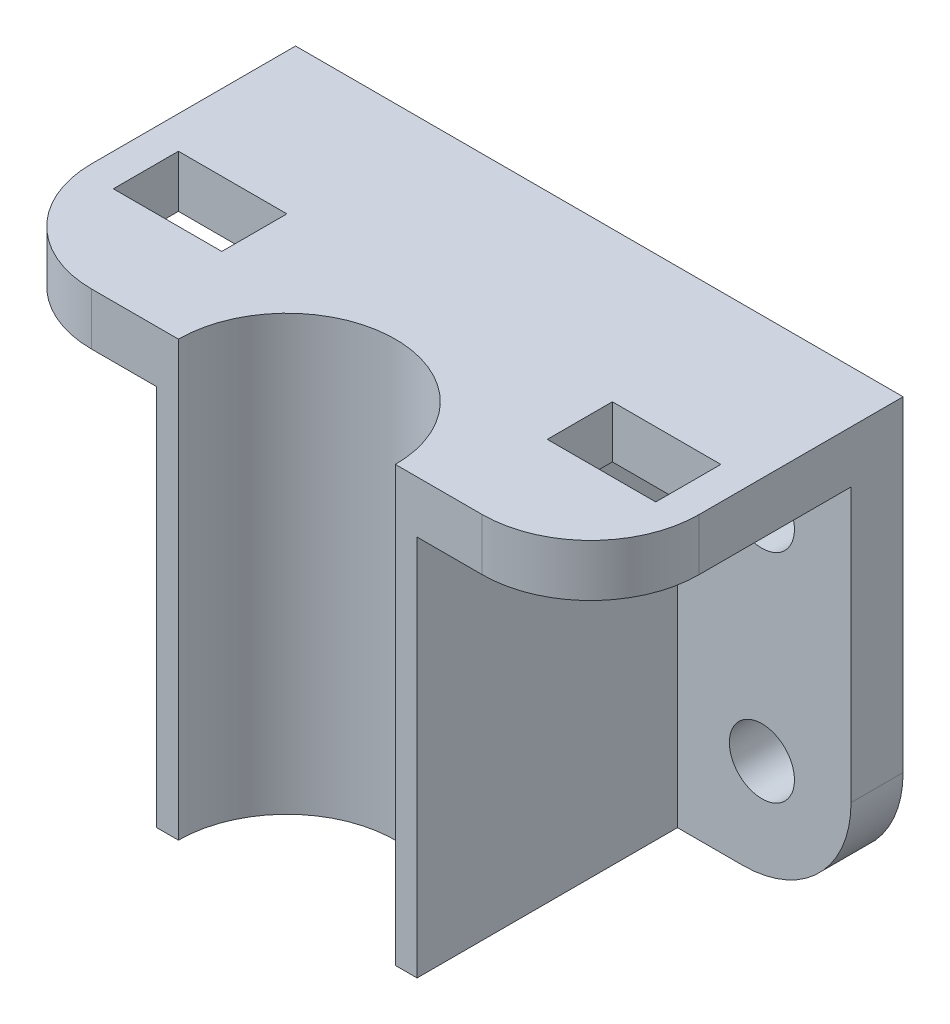
ISO-10303-21;
HEADER;
FILE_DESCRIPTION(('STEP AP214'),'2;1');
FILE_NAME('part.step','',(''),(''),'','','');
FILE_SCHEMA(('AUTOMOTIVE_DESIGN { 1 0 10303 214 1 1 1 1 }'));
ENDSEC;
DATA;
#1=APPLICATION_CONTEXT('core data for automotive mechanical design processes');
#2=APPLICATION_PROTOCOL_DEFINITION('international standard','automotive_design',2000,#1);
#3=PRODUCT_CONTEXT('',#1,'mechanical');
#4=PRODUCT('Part','Part','',(#3));
#5=PRODUCT_RELATED_PRODUCT_CATEGORY('part','',(#4));
#6=PRODUCT_DEFINITION_FORMATION('','',#4);
#7=PRODUCT_DEFINITION_CONTEXT('part definition',#1,'design');
#8=PRODUCT_DEFINITION('design','',#6,#7);
#9=PRODUCT_DEFINITION_SHAPE('','',#8);
#10=(LENGTH_UNIT() NAMED_UNIT(*) SI_UNIT(.MILLI.,.METRE.));
#11=(NAMED_UNIT(*) PLANE_ANGLE_UNIT() SI_UNIT($,.RADIAN.));
#12=(NAMED_UNIT(*) SI_UNIT($,.STERADIAN.) SOLID_ANGLE_UNIT());
#13=UNCERTAINTY_MEASURE_WITH_UNIT(LENGTH_MEASURE(1.E-05),#10,'distance_accuracy_value','');
#14=(GEOMETRIC_REPRESENTATION_CONTEXT(3) GLOBAL_UNCERTAINTY_ASSIGNED_CONTEXT((#13)) GLOBAL_UNIT_ASSIGNED_CONTEXT((#10,
#11,#12)) REPRESENTATION_CONTEXT('',''));
#15=CARTESIAN_POINT('',(0.,0.,0.));
#16=DIRECTION('',(0.,0.,1.));
#17=DIRECTION('',(1.,0.,0.));
#18=AXIS2_PLACEMENT_3D('',#15,#16,#17);
#19=CARTESIAN_POINT('',(115.,-12.,72.));
#20=DIRECTION('',(0.,0.,1.));
#21=DIRECTION('',(1.,0.,0.));
#22=AXIS2_PLACEMENT_3D('',#19,#20,#21);
#23=PLANE('',#22);
#24=DIRECTION('',(0.,1.,0.));
#25=VECTOR('',#24,1.);
#26=CARTESIAN_POINT('',(45.0000000000001,-100.,72.));
#27=LINE('',#26,#25);
#28=CARTESIAN_POINT('',(45.0000000000001,-100.,72.));
#29=VERTEX_POINT('',#28);
#30=CARTESIAN_POINT('',(45.0000000000001,0.,72.));
#31=VERTEX_POINT('',#30);
#32=EDGE_CURVE('E303',#29,#31,#27,.T.);
#33=ORIENTED_EDGE('',*,*,#32,.T.);
#34=DIRECTION('',(1.,0.,0.));
#35=VECTOR('',#34,1.);
#36=CARTESIAN_POINT('',(115.,0.,72.));
#37=LINE('',#36,#35);
#38=CARTESIAN_POINT('',(25.,0.,72.));
#39=VERTEX_POINT('',#38);
#40=EDGE_CURVE('E336',#39,#31,#37,.T.);
#41=ORIENTED_EDGE('',*,*,#40,.F.);
#42=DIRECTION('',(0.,1.,0.));
#43=VECTOR('',#42,1.);
#44=CARTESIAN_POINT('',(25.,-12.,72.));
#45=LINE('',#44,#43);
#46=CARTESIAN_POINT('',(25.,-12.,72.));
#47=VERTEX_POINT('',#46);
#48=EDGE_CURVE('E351',#47,#39,#45,.T.);
#49=ORIENTED_EDGE('',*,*,#48,.F.);
#50=DIRECTION('',(1.,0.,0.));
#51=VECTOR('',#50,1.);
#52=CARTESIAN_POINT('',(115.,-12.,72.));
#53=LINE('',#52,#51);
#54=CARTESIAN_POINT('',(40.0000000000001,-12.,72.));
#55=VERTEX_POINT('',#54);
#56=EDGE_CURVE('E323',#47,#55,#53,.T.);
#57=ORIENTED_EDGE('',*,*,#56,.T.);
#58=DIRECTION('',(0.,1.,0.));
#59=VECTOR('',#58,1.);
#60=CARTESIAN_POINT('',(40.0000000000001,-100.,72.));
#61=LINE('',#60,#59);
#62=CARTESIAN_POINT('',(40.0000000000001,-100.,72.));
#63=VERTEX_POINT('',#62);
#64=EDGE_CURVE('E297',#63,#55,#61,.T.);
#65=ORIENTED_EDGE('',*,*,#64,.F.);
#66=DIRECTION('',(-1.,0.,0.));
#67=VECTOR('',#66,1.);
#68=CARTESIAN_POINT('',(45.0000000000001,-100.,72.));
#69=LINE('',#68,#67);
#70=EDGE_CURVE('E289',#29,#63,#69,.T.);
#71=ORIENTED_EDGE('',*,*,#70,.F.);
#72=EDGE_LOOP('',(#33,#41,#49,#57,#65,#71));
#73=FACE_BOUND('',#72,.T.);
#74=ADVANCED_FACE('F44',(#73),#23,.T.);
#75=CARTESIAN_POINT('',(115.,-75.,12.));
#76=DIRECTION('',(0.,0.,1.));
#77=DIRECTION('',(1.,0.,0.));
#78=AXIS2_PLACEMENT_3D('',#75,#76,#77);
#79=PLANE('',#78);
#80=CARTESIAN_POINT('',(119.4631545479,-27.,12.));
#81=DIRECTION('',(0.,0.,1.));
#82=DIRECTION('',(1.,0.,0.));
#83=AXIS2_PLACEMENT_3D('',#80,#81,#82);
#84=CIRCLE('',#83,7.49999999999998);
#85=CARTESIAN_POINT('',(126.9631545479,-27.,12.));
#86=VERTEX_POINT('',#85);
#87=EDGE_CURVE('E567',#86,#86,#84,.T.);
#88=ORIENTED_EDGE('',*,*,#87,.F.);
#89=EDGE_LOOP('',(#88));
#90=FACE_BOUND('',#89,.T.);
#91=CARTESIAN_POINT('',(119.4631545479,-77.,12.));
#92=DIRECTION('',(0.,0.,1.));
#93=DIRECTION('',(1.,0.,0.));
#94=AXIS2_PLACEMENT_3D('',#91,#92,#93);
#95=CIRCLE('',#94,7.50000000000001);
#96=CARTESIAN_POINT('',(126.9631545479,-77.,12.));
#97=VERTEX_POINT('',#96);
#98=EDGE_CURVE('E230',#97,#97,#95,.T.);
#99=ORIENTED_EDGE('',*,*,#98,.F.);
#100=EDGE_LOOP('',(#99));
#101=FACE_BOUND('',#100,.T.);
#102=DIRECTION('',(-1.,0.,0.));
#103=VECTOR('',#102,1.);
#104=CARTESIAN_POINT('',(140.,-12.,12.));
#105=LINE('',#104,#103);
#106=CARTESIAN_POINT('',(140.,-12.,12.));
#107=VERTEX_POINT('',#106);
#108=CARTESIAN_POINT('',(100.,-12.,12.));
#109=VERTEX_POINT('',#108);
#110=EDGE_CURVE('E313',#107,#109,#105,.T.);
#111=ORIENTED_EDGE('',*,*,#110,.T.);
#112=DIRECTION('',(0.,1.,0.));
#113=VECTOR('',#112,1.);
#114=CARTESIAN_POINT('',(100.,-100.,12.));
#115=LINE('',#114,#113);
#116=CARTESIAN_POINT('',(100.,-100.,12.));
#117=VERTEX_POINT('',#116);
#118=EDGE_CURVE('E309',#117,#109,#115,.T.);
#119=ORIENTED_EDGE('',*,*,#118,.F.);
#120=DIRECTION('',(1.,0.,0.));
#121=VECTOR('',#120,1.);
#122=CARTESIAN_POINT('',(25.,-100.,12.));
#123=LINE('',#122,#121);
#124=CARTESIAN_POINT('',(115.,-100.,12.));
#125=VERTEX_POINT('',#124);
#126=EDGE_CURVE('E359',#117,#125,#123,.T.);
#127=ORIENTED_EDGE('',*,*,#126,.T.);
#128=CARTESIAN_POINT('',(115.,-75.,12.));
#129=DIRECTION('',(0.,0.,1.));
#130=DIRECTION('',(1.,0.,0.));
#131=AXIS2_PLACEMENT_3D('',#128,#129,#130);
#132=CIRCLE('',#131,25.);
#133=CARTESIAN_POINT('',(140.,-75.,12.));
#134=VERTEX_POINT('',#133);
#135=EDGE_CURVE('E361',#125,#134,#132,.T.);
#136=ORIENTED_EDGE('',*,*,#135,.T.);
#137=DIRECTION('',(0.,1.,0.));
#138=VECTOR('',#137,1.);
#139=CARTESIAN_POINT('',(140.,0.,12.));
#140=LINE('',#139,#138);
#141=EDGE_CURVE('E362',#134,#107,#140,.T.);
#142=ORIENTED_EDGE('',*,*,#141,.T.);
#143=EDGE_LOOP('',(#111,#119,#127,#136,#142));
#144=FACE_BOUND('',#143,.T.);
#145=ADVANCED_FACE('F416',(#90,#101,#144),#79,.T.);
#146=CARTESIAN_POINT('',(19.128084721305,-27.,12.));
#147=DIRECTION('',(0.,0.,1.));
#148=DIRECTION('',(1.,0.,0.));
#149=AXIS2_PLACEMENT_3D('',#146,#147,#148);
#150=CIRCLE('',#149,7.5);
#151=CARTESIAN_POINT('',(26.628084721305,-27.,12.));
#152=VERTEX_POINT('',#151);
#153=EDGE_CURVE('E558',#152,#152,#150,.T.);
#154=ORIENTED_EDGE('',*,*,#153,.F.);
#155=EDGE_LOOP('',(#154));
#156=FACE_BOUND('',#155,.T.);
#157=CARTESIAN_POINT('',(19.128084721305,-77.,12.));
#158=DIRECTION('',(0.,0.,1.));
#159=DIRECTION('',(1.,0.,0.));
#160=AXIS2_PLACEMENT_3D('',#157,#158,#159);
#161=CIRCLE('',#160,7.5);
#162=CARTESIAN_POINT('',(26.628084721305,-77.,12.));
#163=VERTEX_POINT('',#162);
#164=EDGE_CURVE('E565',#163,#163,#161,.T.);
#165=ORIENTED_EDGE('',*,*,#164,.F.);
#166=EDGE_LOOP('',(#165));
#167=FACE_BOUND('',#166,.T.);
#168=CARTESIAN_POINT('',(25.,-100.,12.));
#169=VERTEX_POINT('',#168);
#170=CARTESIAN_POINT('',(40.0000000000001,-100.,12.));
#171=VERTEX_POINT('',#170);
#172=EDGE_CURVE('E363',#169,#171,#123,.T.);
#173=ORIENTED_EDGE('',*,*,#172,.T.);
#174=DIRECTION('',(0.,1.,0.));
#175=VECTOR('',#174,1.);
#176=CARTESIAN_POINT('',(40.0000000000001,-100.,12.));
#177=LINE('',#176,#175);
#178=CARTESIAN_POINT('',(40.0000000000001,-12.,12.));
#179=VERTEX_POINT('',#178);
#180=EDGE_CURVE('E291',#171,#179,#177,.T.);
#181=ORIENTED_EDGE('',*,*,#180,.T.);
#182=CARTESIAN_POINT('',(0.,-12.,12.));
#183=VERTEX_POINT('',#182);
#184=EDGE_CURVE('E319',#179,#183,#105,.T.);
#185=ORIENTED_EDGE('',*,*,#184,.T.);
#186=DIRECTION('',(0.,-1.,0.));
#187=VECTOR('',#186,1.);
#188=CARTESIAN_POINT('',(0.,0.,12.));
#189=LINE('',#188,#187);
#190=CARTESIAN_POINT('',(0.,-75.,12.));
#191=VERTEX_POINT('',#190);
#192=EDGE_CURVE('E355',#183,#191,#189,.T.);
#193=ORIENTED_EDGE('',*,*,#192,.T.);
#194=CARTESIAN_POINT('',(25.,-75.,12.));
#195=DIRECTION('',(0.,0.,1.));
#196=DIRECTION('',(1.,0.,0.));
#197=AXIS2_PLACEMENT_3D('',#194,#195,#196);
#198=CIRCLE('',#197,25.);
#199=EDGE_CURVE('E357',#191,#169,#198,.T.);
#200=ORIENTED_EDGE('',*,*,#199,.T.);
#201=EDGE_LOOP('',(#173,#181,#185,#193,#200));
#202=FACE_BOUND('',#201,.T.);
#203=ADVANCED_FACE('F441',(#156,#167,#202),#79,.T.);
#204=CARTESIAN_POINT('',(25.,-12.,47.));
#205=DIRECTION('',(0.,1.,0.));
#206=DIRECTION('',(0.,0.,1.));
#207=AXIS2_PLACEMENT_3D('',#204,#205,#206);
#208=PLANE('',#207);
#209=DIRECTION('',(1.,0.,0.));
#210=VECTOR('',#209,1.);
#211=CARTESIAN_POINT('',(107.5,-12.,34.5));
#212=LINE('',#211,#210);
#213=CARTESIAN_POINT('',(107.5,-12.,34.5));
#214=VERTEX_POINT('',#213);
#215=CARTESIAN_POINT('',(132.5,-12.,34.5));
#216=VERTEX_POINT('',#215);
#217=EDGE_CURVE('E262',#214,#216,#212,.T.);
#218=ORIENTED_EDGE('',*,*,#217,.F.);
#219=DIRECTION('',(0.,0.,-1.));
#220=VECTOR('',#219,1.);
#221=CARTESIAN_POINT('',(107.5,-12.,49.5));
#222=LINE('',#221,#220);
#223=CARTESIAN_POINT('',(107.5,-12.,49.5));
#224=VERTEX_POINT('',#223);
#225=EDGE_CURVE('E245',#224,#214,#222,.T.);
#226=ORIENTED_EDGE('',*,*,#225,.F.);
#227=DIRECTION('',(-1.,0.,0.));
#228=VECTOR('',#227,1.);
#229=CARTESIAN_POINT('',(107.5,-12.,49.5));
#230=LINE('',#229,#228);
#231=CARTESIAN_POINT('',(132.5,-12.,49.5));
#232=VERTEX_POINT('',#231);
#233=EDGE_CURVE('E249',#232,#224,#230,.T.);
#234=ORIENTED_EDGE('',*,*,#233,.F.);
#235=DIRECTION('',(0.,0.,1.));
#236=VECTOR('',#235,1.);
#237=CARTESIAN_POINT('',(132.5,-12.,49.5));
#238=LINE('',#237,#236);
#239=EDGE_CURVE('E261',#216,#232,#238,.T.);
#240=ORIENTED_EDGE('',*,*,#239,.F.);
#241=EDGE_LOOP('',(#218,#226,#234,#240));
#242=FACE_BOUND('',#241,.T.);
#243=DIRECTION('',(0.,0.,1.));
#244=VECTOR('',#243,1.);
#245=CARTESIAN_POINT('',(100.,-12.,72.));
#246=LINE('',#245,#244);
#247=CARTESIAN_POINT('',(100.,-12.,72.));
#248=VERTEX_POINT('',#247);
#249=EDGE_CURVE('E278',#109,#248,#246,.T.);
#250=ORIENTED_EDGE('',*,*,#249,.F.);
#251=ORIENTED_EDGE('',*,*,#110,.F.);
#252=DIRECTION('',(0.,0.,-1.));
#253=VECTOR('',#252,1.);
#254=CARTESIAN_POINT('',(140.,-12.,12.));
#255=LINE('',#254,#253);
#256=CARTESIAN_POINT('',(140.,-12.,47.));
#257=VERTEX_POINT('',#256);
#258=EDGE_CURVE('E331',#257,#107,#255,.T.);
#259=ORIENTED_EDGE('',*,*,#258,.F.);
#260=CARTESIAN_POINT('',(115.,-12.,47.));
#261=DIRECTION('',(0.,1.,0.));
#262=DIRECTION('',(0.,0.,1.));
#263=AXIS2_PLACEMENT_3D('',#260,#261,#262);
#264=CIRCLE('',#263,25.);
#265=CARTESIAN_POINT('',(115.,-12.,72.));
#266=VERTEX_POINT('',#265);
#267=EDGE_CURVE('E330',#266,#257,#264,.T.);
#268=ORIENTED_EDGE('',*,*,#267,.F.);
#269=EDGE_CURVE('E321',#248,#266,#53,.T.);
#270=ORIENTED_EDGE('',*,*,#269,.F.);
#271=EDGE_LOOP('',(#250,#251,#259,#268,#270));
#272=FACE_BOUND('',#271,.T.);
#273=ADVANCED_FACE('F457',(#242,#272),#208,.F.);
#274=DIRECTION('',(1.,0.,0.));
#275=VECTOR('',#274,1.);
#276=CARTESIAN_POINT('',(7.5,-12.,34.5));
#277=LINE('',#276,#275);
#278=CARTESIAN_POINT('',(7.5,-12.,34.5));
#279=VERTEX_POINT('',#278);
#280=CARTESIAN_POINT('',(32.5,-12.,34.5));
#281=VERTEX_POINT('',#280);
#282=EDGE_CURVE('E232',#279,#281,#277,.T.);
#283=ORIENTED_EDGE('',*,*,#282,.F.);
#284=DIRECTION('',(0.,0.,-1.));
#285=VECTOR('',#284,1.);
#286=CARTESIAN_POINT('',(7.5,-12.,49.5));
#287=LINE('',#286,#285);
#288=CARTESIAN_POINT('',(7.5,-12.,49.5));
#289=VERTEX_POINT('',#288);
#290=EDGE_CURVE('E58',#289,#279,#287,.T.);
#291=ORIENTED_EDGE('',*,*,#290,.F.);
#292=DIRECTION('',(-1.,0.,0.));
#293=VECTOR('',#292,1.);
#294=CARTESIAN_POINT('',(7.5,-12.,49.5));
#295=LINE('',#294,#293);
#296=CARTESIAN_POINT('',(32.5,-12.,49.5));
#297=VERTEX_POINT('',#296);
#298=EDGE_CURVE('E224',#297,#289,#295,.T.);
#299=ORIENTED_EDGE('',*,*,#298,.F.);
#300=DIRECTION('',(0.,0.,1.));
#301=VECTOR('',#300,1.);
#302=CARTESIAN_POINT('',(32.5,-12.,49.5));
#303=LINE('',#302,#301);
#304=EDGE_CURVE('E228',#281,#297,#303,.T.);
#305=ORIENTED_EDGE('',*,*,#304,.F.);
#306=EDGE_LOOP('',(#283,#291,#299,#305));
#307=FACE_BOUND('',#306,.T.);
#308=DIRECTION('',(0.,0.,-1.));
#309=VECTOR('',#308,1.);
#310=CARTESIAN_POINT('',(40.0000000000001,-12.,72.));
#311=LINE('',#310,#309);
#312=EDGE_CURVE('E281',#55,#179,#311,.T.);
#313=ORIENTED_EDGE('',*,*,#312,.F.);
#314=ORIENTED_EDGE('',*,*,#56,.F.);
#315=CARTESIAN_POINT('',(25.,-12.,47.));
#316=DIRECTION('',(0.,1.,0.));
#317=DIRECTION('',(0.,0.,1.));
#318=AXIS2_PLACEMENT_3D('',#315,#316,#317);
#319=CIRCLE('',#318,25.);
#320=CARTESIAN_POINT('',(0.,-12.,47.));
#321=VERTEX_POINT('',#320);
#322=EDGE_CURVE('E322',#321,#47,#319,.T.);
#323=ORIENTED_EDGE('',*,*,#322,.F.);
#324=DIRECTION('',(0.,0.,1.));
#325=VECTOR('',#324,1.);
#326=CARTESIAN_POINT('',(0.,-12.,12.));
#327=LINE('',#326,#325);
#328=EDGE_CURVE('E320',#183,#321,#327,.T.);
#329=ORIENTED_EDGE('',*,*,#328,.F.);
#330=ORIENTED_EDGE('',*,*,#184,.F.);
#331=EDGE_LOOP('',(#313,#314,#323,#329,#330));
#332=FACE_BOUND('',#331,.T.);
#333=ADVANCED_FACE('F450',(#307,#332),#208,.F.);
#334=CARTESIAN_POINT('',(0.,0.,12.));
#335=DIRECTION('',(0.,-1.,0.));
#336=DIRECTION('',(0.,0.,-1.));
#337=AXIS2_PLACEMENT_3D('',#334,#335,#336);
#338=PLANE('',#337);
#339=DIRECTION('',(-1.,0.,0.));
#340=VECTOR('',#339,1.);
#341=CARTESIAN_POINT('',(7.5,0.,49.5));
#342=LINE('',#341,#340);
#343=CARTESIAN_POINT('',(32.5,0.,49.5));
#344=VERTEX_POINT('',#343);
#345=CARTESIAN_POINT('',(7.5,0.,49.5));
#346=VERTEX_POINT('',#345);
#347=EDGE_CURVE('E211',#344,#346,#342,.T.);
#348=ORIENTED_EDGE('',*,*,#347,.T.);
#349=DIRECTION('',(0.,0.,-1.));
#350=VECTOR('',#349,1.);
#351=CARTESIAN_POINT('',(7.5,0.,49.5));
#352=LINE('',#351,#350);
#353=CARTESIAN_POINT('',(7.5,0.,34.5));
#354=VERTEX_POINT('',#353);
#355=EDGE_CURVE('E206',#346,#354,#352,.T.);
#356=ORIENTED_EDGE('',*,*,#355,.T.);
#357=DIRECTION('',(1.,0.,0.));
#358=VECTOR('',#357,1.);
#359=CARTESIAN_POINT('',(7.5,0.,34.5));
#360=LINE('',#359,#358);
#361=CARTESIAN_POINT('',(32.5,0.,34.5));
#362=VERTEX_POINT('',#361);
#363=EDGE_CURVE('E219',#354,#362,#360,.T.);
#364=ORIENTED_EDGE('',*,*,#363,.T.);
#365=DIRECTION('',(0.,0.,1.));
#366=VECTOR('',#365,1.);
#367=CARTESIAN_POINT('',(32.5,0.,49.5));
#368=LINE('',#367,#366);
#369=EDGE_CURVE('E70',#362,#344,#368,.T.);
#370=ORIENTED_EDGE('',*,*,#369,.T.);
#371=EDGE_LOOP('',(#348,#356,#364,#370));
#372=FACE_BOUND('',#371,.T.);
#373=DIRECTION('',(-1.,0.,0.));
#374=VECTOR('',#373,1.);
#375=CARTESIAN_POINT('',(107.5,0.,49.5));
#376=LINE('',#375,#374);
#377=CARTESIAN_POINT('',(132.5,0.,49.5));
#378=VERTEX_POINT('',#377);
#379=CARTESIAN_POINT('',(107.5,0.,49.5));
#380=VERTEX_POINT('',#379);
#381=EDGE_CURVE('E257',#378,#380,#376,.T.);
#382=ORIENTED_EDGE('',*,*,#381,.T.);
#383=DIRECTION('',(0.,0.,-1.));
#384=VECTOR('',#383,1.);
#385=CARTESIAN_POINT('',(107.5,0.,49.5));
#386=LINE('',#385,#384);
#387=CARTESIAN_POINT('',(107.5,0.,34.5));
#388=VERTEX_POINT('',#387);
#389=EDGE_CURVE('E246',#380,#388,#386,.T.);
#390=ORIENTED_EDGE('',*,*,#389,.T.);
#391=DIRECTION('',(1.,0.,0.));
#392=VECTOR('',#391,1.);
#393=CARTESIAN_POINT('',(107.5,0.,34.5));
#394=LINE('',#393,#392);
#395=CARTESIAN_POINT('',(132.5,0.,34.5));
#396=VERTEX_POINT('',#395);
#397=EDGE_CURVE('E248',#388,#396,#394,.T.);
#398=ORIENTED_EDGE('',*,*,#397,.T.);
#399=DIRECTION('',(0.,0.,1.));
#400=VECTOR('',#399,1.);
#401=CARTESIAN_POINT('',(132.5,0.,49.5));
#402=LINE('',#401,#400);
#403=EDGE_CURVE('E254',#396,#378,#402,.T.);
#404=ORIENTED_EDGE('',*,*,#403,.T.);
#405=EDGE_LOOP('',(#382,#390,#398,#404));
#406=FACE_BOUND('',#405,.T.);
#407=ORIENTED_EDGE('',*,*,#40,.T.);
#408=CARTESIAN_POINT('',(70.0000000000001,0.,72.));
#409=DIRECTION('',(0.,-1.,0.));
#410=DIRECTION('',(0.,0.,-1.));
#411=AXIS2_PLACEMENT_3D('',#408,#409,#410);
#412=CIRCLE('',#411,25.);
#413=CARTESIAN_POINT('',(95.0000000000002,0.,72.));
#414=VERTEX_POINT('',#413);
#415=EDGE_CURVE('E272',#31,#414,#412,.T.);
#416=ORIENTED_EDGE('',*,*,#415,.T.);
#417=CARTESIAN_POINT('',(115.,0.,72.));
#418=VERTEX_POINT('',#417);
#419=EDGE_CURVE('E340',#414,#418,#37,.T.);
#420=ORIENTED_EDGE('',*,*,#419,.T.);
#421=CARTESIAN_POINT('',(115.,0.,47.));
#422=DIRECTION('',(0.,1.,0.));
#423=DIRECTION('',(0.,0.,1.));
#424=AXIS2_PLACEMENT_3D('',#421,#422,#423);
#425=CIRCLE('',#424,25.);
#426=CARTESIAN_POINT('',(140.,0.,47.));
#427=VERTEX_POINT('',#426);
#428=EDGE_CURVE('E342',#418,#427,#425,.T.);
#429=ORIENTED_EDGE('',*,*,#428,.T.);
#430=DIRECTION('',(0.,0.,-1.));
#431=VECTOR('',#430,1.);
#432=CARTESIAN_POINT('',(140.,0.,12.));
#433=LINE('',#432,#431);
#434=CARTESIAN_POINT('',(140.,0.,0.));
#435=VERTEX_POINT('',#434);
#436=EDGE_CURVE('E368',#427,#435,#433,.T.);
#437=ORIENTED_EDGE('',*,*,#436,.T.);
#438=DIRECTION('',(-1.,0.,0.));
#439=VECTOR('',#438,1.);
#440=CARTESIAN_POINT('',(0.,0.,0.));
#441=LINE('',#440,#439);
#442=CARTESIAN_POINT('',(0.,0.,0.));
#443=VERTEX_POINT('',#442);
#444=EDGE_CURVE('E349',#435,#443,#441,.T.);
#445=ORIENTED_EDGE('',*,*,#444,.T.);
#446=DIRECTION('',(0.,0.,-1.));
#447=VECTOR('',#446,1.);
#448=CARTESIAN_POINT('',(0.,0.,12.));
#449=LINE('',#448,#447);
#450=CARTESIAN_POINT('',(0.,0.,47.));
#451=VERTEX_POINT('',#450);
#452=EDGE_CURVE('E11',#451,#443,#449,.T.);
#453=ORIENTED_EDGE('',*,*,#452,.F.);
#454=CARTESIAN_POINT('',(25.,0.,47.));
#455=DIRECTION('',(0.,1.,0.));
#456=DIRECTION('',(0.,0.,1.));
#457=AXIS2_PLACEMENT_3D('',#454,#455,#456);
#458=CIRCLE('',#457,25.);
#459=EDGE_CURVE('E312',#451,#39,#458,.T.);
#460=ORIENTED_EDGE('',*,*,#459,.T.);
#461=EDGE_LOOP('',(#407,#416,#420,#429,#437,#445,#453,#460));
#462=FACE_BOUND('',#461,.T.);
#463=ADVANCED_FACE('F50',(#372,#406,#462),#338,.F.);
#464=CARTESIAN_POINT('',(0.,0.,12.));
#465=DIRECTION('',(1.,0.,0.));
#466=DIRECTION('',(0.,0.,-1.));
#467=AXIS2_PLACEMENT_3D('',#464,#465,#466);
#468=PLANE('',#467);
#469=DIRECTION('',(0.,-1.,0.));
#470=VECTOR('',#469,1.);
#471=CARTESIAN_POINT('',(0.,0.,0.));
#472=LINE('',#471,#470);
#473=CARTESIAN_POINT('',(0.,-75.,0.));
#474=VERTEX_POINT('',#473);
#475=EDGE_CURVE('E371',#443,#474,#472,.T.);
#476=ORIENTED_EDGE('',*,*,#475,.T.);
#477=DIRECTION('',(0.,0.,-1.));
#478=VECTOR('',#477,1.);
#479=CARTESIAN_POINT('',(0.,-75.,12.));
#480=LINE('',#479,#478);
#481=EDGE_CURVE('E52',#191,#474,#480,.T.);
#482=ORIENTED_EDGE('',*,*,#481,.F.);
#483=ORIENTED_EDGE('',*,*,#192,.F.);
#484=ORIENTED_EDGE('',*,*,#328,.T.);
#485=DIRECTION('',(0.,1.,0.));
#486=VECTOR('',#485,1.);
#487=CARTESIAN_POINT('',(0.,-12.,47.));
#488=LINE('',#487,#486);
#489=EDGE_CURVE('E333',#321,#451,#488,.T.);
#490=ORIENTED_EDGE('',*,*,#489,.T.);
#491=ORIENTED_EDGE('',*,*,#452,.T.);
#492=EDGE_LOOP('',(#476,#482,#483,#484,#490,#491));
#493=FACE_BOUND('',#492,.T.);
#494=ADVANCED_FACE('F442',(#493),#468,.F.);
#495=CARTESIAN_POINT('',(25.,-75.,12.));
#496=DIRECTION('',(0.,0.,-1.));
#497=DIRECTION('',(-1.,0.,0.));
#498=AXIS2_PLACEMENT_3D('',#495,#496,#497);
#499=CYLINDRICAL_SURFACE('',#498,25.);
#500=CARTESIAN_POINT('',(25.,-75.,0.));
#501=DIRECTION('',(0.,0.,1.));
#502=DIRECTION('',(1.,0.,0.));
#503=AXIS2_PLACEMENT_3D('',#500,#501,#502);
#504=CIRCLE('',#503,25.);
#505=CARTESIAN_POINT('',(25.,-100.,0.));
#506=VERTEX_POINT('',#505);
#507=EDGE_CURVE('E373',#474,#506,#504,.T.);
#508=ORIENTED_EDGE('',*,*,#507,.T.);
#509=DIRECTION('',(0.,0.,-1.));
#510=VECTOR('',#509,1.);
#511=CARTESIAN_POINT('',(25.,-100.,12.));
#512=LINE('',#511,#510);
#513=EDGE_CURVE('E389',#169,#506,#512,.T.);
#514=ORIENTED_EDGE('',*,*,#513,.F.);
#515=ORIENTED_EDGE('',*,*,#199,.F.);
#516=ORIENTED_EDGE('',*,*,#481,.T.);
#517=EDGE_LOOP('',(#508,#514,#515,#516));
#518=FACE_BOUND('',#517,.T.);
#519=ADVANCED_FACE('F393',(#518),#499,.T.);
#520=CARTESIAN_POINT('',(25.,-100.,12.));
#521=DIRECTION('',(0.,1.,0.));
#522=DIRECTION('',(0.,0.,1.));
#523=AXIS2_PLACEMENT_3D('',#520,#521,#522);
#524=PLANE('',#523);
#525=DIRECTION('',(1.,0.,0.));
#526=VECTOR('',#525,1.);
#527=CARTESIAN_POINT('',(25.,-100.,0.));
#528=LINE('',#527,#526);
#529=CARTESIAN_POINT('',(115.,-100.,0.));
#530=VERTEX_POINT('',#529);
#531=EDGE_CURVE('E374',#506,#530,#528,.T.);
#532=ORIENTED_EDGE('',*,*,#531,.T.);
#533=DIRECTION('',(0.,0.,-1.));
#534=VECTOR('',#533,1.);
#535=CARTESIAN_POINT('',(115.,-100.,12.));
#536=LINE('',#535,#534);
#537=EDGE_CURVE('E383',#125,#530,#536,.T.);
#538=ORIENTED_EDGE('',*,*,#537,.F.);
#539=ORIENTED_EDGE('',*,*,#126,.F.);
#540=DIRECTION('',(0.,0.,1.));
#541=VECTOR('',#540,1.);
#542=CARTESIAN_POINT('',(100.,-100.,72.));
#543=LINE('',#542,#541);
#544=CARTESIAN_POINT('',(100.,-100.,72.));
#545=VERTEX_POINT('',#544);
#546=EDGE_CURVE('E282',#117,#545,#543,.T.);
#547=ORIENTED_EDGE('',*,*,#546,.T.);
#548=DIRECTION('',(-1.,0.,0.));
#549=VECTOR('',#548,1.);
#550=CARTESIAN_POINT('',(95.0000000000002,-100.,72.));
#551=LINE('',#550,#549);
#552=CARTESIAN_POINT('',(95.0000000000002,-100.,72.));
#553=VERTEX_POINT('',#552);
#554=EDGE_CURVE('E285',#545,#553,#551,.T.);
#555=ORIENTED_EDGE('',*,*,#554,.T.);
#556=CARTESIAN_POINT('',(70.0000000000001,-100.,72.));
#557=DIRECTION('',(0.,1.,0.));
#558=DIRECTION('',(0.,0.,-1.));
#559=AXIS2_PLACEMENT_3D('',#556,#557,#558);
#560=CIRCLE('',#559,25.);
#561=EDGE_CURVE('E286',#553,#29,#560,.T.);
#562=ORIENTED_EDGE('',*,*,#561,.T.);
#563=ORIENTED_EDGE('',*,*,#70,.T.);
#564=DIRECTION('',(0.,0.,-1.));
#565=VECTOR('',#564,1.);
#566=CARTESIAN_POINT('',(40.0000000000001,-100.,72.));
#567=LINE('',#566,#565);
#568=EDGE_CURVE('E290',#63,#171,#567,.T.);
#569=ORIENTED_EDGE('',*,*,#568,.T.);
#570=ORIENTED_EDGE('',*,*,#172,.F.);
#571=ORIENTED_EDGE('',*,*,#513,.T.);
#572=EDGE_LOOP('',(#532,#538,#539,#547,#555,#562,#563,#569,#570,#571));
#573=FACE_BOUND('',#572,.T.);
#574=ADVANCED_FACE('F410',(#573),#524,.F.);
#575=CARTESIAN_POINT('',(115.,-75.,12.));
#576=DIRECTION('',(0.,0.,-1.));
#577=DIRECTION('',(-1.,0.,0.));
#578=AXIS2_PLACEMENT_3D('',#575,#576,#577);
#579=CYLINDRICAL_SURFACE('',#578,25.);
#580=CARTESIAN_POINT('',(115.,-75.,0.));
#581=DIRECTION('',(0.,0.,1.));
#582=DIRECTION('',(1.,0.,0.));
#583=AXIS2_PLACEMENT_3D('',#580,#581,#582);
#584=CIRCLE('',#583,25.);
#585=CARTESIAN_POINT('',(140.,-75.,0.));
#586=VERTEX_POINT('',#585);
#587=EDGE_CURVE('E380',#530,#586,#584,.T.);
#588=ORIENTED_EDGE('',*,*,#587,.T.);
#589=DIRECTION('',(0.,0.,-1.));
#590=VECTOR('',#589,1.);
#591=CARTESIAN_POINT('',(140.,-75.,12.));
#592=LINE('',#591,#590);
#593=EDGE_CURVE('E385',#134,#586,#592,.T.);
#594=ORIENTED_EDGE('',*,*,#593,.F.);
#595=ORIENTED_EDGE('',*,*,#135,.F.);
#596=ORIENTED_EDGE('',*,*,#537,.T.);
#597=EDGE_LOOP('',(#588,#594,#595,#596));
#598=FACE_BOUND('',#597,.T.);
#599=ADVANCED_FACE('F414',(#598),#579,.T.);
#600=CARTESIAN_POINT('',(140.,0.,12.));
#601=DIRECTION('',(-1.,0.,0.));
#602=DIRECTION('',(0.,0.,1.));
#603=AXIS2_PLACEMENT_3D('',#600,#601,#602);
#604=PLANE('',#603);
#605=DIRECTION('',(0.,1.,0.));
#606=VECTOR('',#605,1.);
#607=CARTESIAN_POINT('',(140.,0.,0.));
#608=LINE('',#607,#606);
#609=EDGE_CURVE('E356',#586,#435,#608,.T.);
#610=ORIENTED_EDGE('',*,*,#609,.T.);
#611=ORIENTED_EDGE('',*,*,#436,.F.);
#612=DIRECTION('',(0.,1.,0.));
#613=VECTOR('',#612,1.);
#614=CARTESIAN_POINT('',(140.,-12.,47.));
#615=LINE('',#614,#613);
#616=EDGE_CURVE('E341',#257,#427,#615,.T.);
#617=ORIENTED_EDGE('',*,*,#616,.F.);
#618=ORIENTED_EDGE('',*,*,#258,.T.);
#619=ORIENTED_EDGE('',*,*,#141,.F.);
#620=ORIENTED_EDGE('',*,*,#593,.T.);
#621=EDGE_LOOP('',(#610,#611,#617,#618,#619,#620));
#622=FACE_BOUND('',#621,.T.);
#623=ADVANCED_FACE('F455',(#622),#604,.F.);
#624=CARTESIAN_POINT('',(115.,-75.,0.));
#625=DIRECTION('',(0.,0.,1.));
#626=DIRECTION('',(1.,0.,0.));
#627=AXIS2_PLACEMENT_3D('',#624,#625,#626);
#628=PLANE('',#627);
#629=CARTESIAN_POINT('',(19.128084721305,-27.,0.));
#630=DIRECTION('',(0.,0.,1.));
#631=DIRECTION('',(1.,0.,0.));
#632=AXIS2_PLACEMENT_3D('',#629,#630,#631);
#633=CIRCLE('',#632,7.5);
#634=CARTESIAN_POINT('',(26.628084721305,-27.,0.));
#635=VERTEX_POINT('',#634);
#636=EDGE_CURVE('E551',#635,#635,#633,.T.);
#637=ORIENTED_EDGE('',*,*,#636,.T.);
#638=EDGE_LOOP('',(#637));
#639=FACE_BOUND('',#638,.T.);
#640=CARTESIAN_POINT('',(19.128084721305,-77.,0.));
#641=DIRECTION('',(0.,0.,1.));
#642=DIRECTION('',(1.,0.,0.));
#643=AXIS2_PLACEMENT_3D('',#640,#641,#642);
#644=CIRCLE('',#643,7.5);
#645=CARTESIAN_POINT('',(26.628084721305,-77.,0.));
#646=VERTEX_POINT('',#645);
#647=EDGE_CURVE('E556',#646,#646,#644,.T.);
#648=ORIENTED_EDGE('',*,*,#647,.T.);
#649=EDGE_LOOP('',(#648));
#650=FACE_BOUND('',#649,.T.);
#651=CARTESIAN_POINT('',(119.4631545479,-27.,0.));
#652=DIRECTION('',(0.,0.,1.));
#653=DIRECTION('',(1.,0.,0.));
#654=AXIS2_PLACEMENT_3D('',#651,#652,#653);
#655=CIRCLE('',#654,7.49999999999998);
#656=CARTESIAN_POINT('',(126.9631545479,-27.,0.));
#657=VERTEX_POINT('',#656);
#658=EDGE_CURVE('E236',#657,#657,#655,.T.);
#659=ORIENTED_EDGE('',*,*,#658,.T.);
#660=EDGE_LOOP('',(#659));
#661=FACE_BOUND('',#660,.T.);
#662=CARTESIAN_POINT('',(119.4631545479,-77.,0.));
#663=DIRECTION('',(0.,0.,1.));
#664=DIRECTION('',(1.,0.,0.));
#665=AXIS2_PLACEMENT_3D('',#662,#663,#664);
#666=CIRCLE('',#665,7.50000000000001);
#667=CARTESIAN_POINT('',(126.9631545479,-77.,0.));
#668=VERTEX_POINT('',#667);
#669=EDGE_CURVE('E571',#668,#668,#666,.T.);
#670=ORIENTED_EDGE('',*,*,#669,.T.);
#671=EDGE_LOOP('',(#670));
#672=FACE_BOUND('',#671,.T.);
#673=ORIENTED_EDGE('',*,*,#444,.F.);
#674=ORIENTED_EDGE('',*,*,#609,.F.);
#675=ORIENTED_EDGE('',*,*,#587,.F.);
#676=ORIENTED_EDGE('',*,*,#531,.F.);
#677=ORIENTED_EDGE('',*,*,#507,.F.);
#678=ORIENTED_EDGE('',*,*,#475,.F.);
#679=EDGE_LOOP('',(#673,#674,#675,#676,#677,#678));
#680=FACE_BOUND('',#679,.T.);
#681=ADVANCED_FACE('F405',(#639,#650,#661,#672,#680),#628,.F.);
#682=CARTESIAN_POINT('',(115.,-12.,47.));
#683=DIRECTION('',(0.,1.,0.));
#684=DIRECTION('',(0.,0.,1.));
#685=AXIS2_PLACEMENT_3D('',#682,#683,#684);
#686=CYLINDRICAL_SURFACE('',#685,25.);
#687=ORIENTED_EDGE('',*,*,#428,.F.);
#688=DIRECTION('',(0.,1.,0.));
#689=VECTOR('',#688,1.);
#690=CARTESIAN_POINT('',(115.,-12.,72.));
#691=LINE('',#690,#689);
#692=EDGE_CURVE('E350',#266,#418,#691,.T.);
#693=ORIENTED_EDGE('',*,*,#692,.F.);
#694=ORIENTED_EDGE('',*,*,#267,.T.);
#695=ORIENTED_EDGE('',*,*,#616,.T.);
#696=EDGE_LOOP('',(#687,#693,#694,#695));
#697=FACE_BOUND('',#696,.T.);
#698=ADVANCED_FACE('F458',(#697),#686,.T.);
#699=ORIENTED_EDGE('',*,*,#419,.F.);
#700=DIRECTION('',(0.,1.,0.));
#701=VECTOR('',#700,1.);
#702=CARTESIAN_POINT('',(95.0000000000002,-100.,72.));
#703=LINE('',#702,#701);
#704=EDGE_CURVE('E304',#553,#414,#703,.T.);
#705=ORIENTED_EDGE('',*,*,#704,.F.);
#706=ORIENTED_EDGE('',*,*,#554,.F.);
#707=DIRECTION('',(0.,1.,0.));
#708=VECTOR('',#707,1.);
#709=CARTESIAN_POINT('',(100.,-100.,72.));
#710=LINE('',#709,#708);
#711=EDGE_CURVE('E310',#545,#248,#710,.T.);
#712=ORIENTED_EDGE('',*,*,#711,.T.);
#713=ORIENTED_EDGE('',*,*,#269,.T.);
#714=ORIENTED_EDGE('',*,*,#692,.T.);
#715=EDGE_LOOP('',(#699,#705,#706,#712,#713,#714));
#716=FACE_BOUND('',#715,.T.);
#717=ADVANCED_FACE('F424',(#716),#23,.T.);
#718=CARTESIAN_POINT('',(25.,-12.,47.));
#719=DIRECTION('',(0.,1.,0.));
#720=DIRECTION('',(0.,0.,1.));
#721=AXIS2_PLACEMENT_3D('',#718,#719,#720);
#722=CYLINDRICAL_SURFACE('',#721,25.);
#723=ORIENTED_EDGE('',*,*,#459,.F.);
#724=ORIENTED_EDGE('',*,*,#489,.F.);
#725=ORIENTED_EDGE('',*,*,#322,.T.);
#726=ORIENTED_EDGE('',*,*,#48,.T.);
#727=EDGE_LOOP('',(#723,#724,#725,#726));
#728=FACE_BOUND('',#727,.T.);
#729=ADVANCED_FACE('F446',(#728),#722,.T.);
#730=CARTESIAN_POINT('',(100.,-100.,72.));
#731=DIRECTION('',(-1.,0.,0.));
#732=DIRECTION('',(0.,0.,1.));
#733=AXIS2_PLACEMENT_3D('',#730,#731,#732);
#734=PLANE('',#733);
#735=ORIENTED_EDGE('',*,*,#249,.T.);
#736=ORIENTED_EDGE('',*,*,#711,.F.);
#737=ORIENTED_EDGE('',*,*,#546,.F.);
#738=ORIENTED_EDGE('',*,*,#118,.T.);
#739=EDGE_LOOP('',(#735,#736,#737,#738));
#740=FACE_BOUND('',#739,.T.);
#741=ADVANCED_FACE('F420',(#740),#734,.F.);
#742=CARTESIAN_POINT('',(70.0000000000001,-100.,72.));
#743=DIRECTION('',(0.,1.,0.));
#744=DIRECTION('',(0.,0.,1.));
#745=AXIS2_PLACEMENT_3D('',#742,#743,#744);
#746=CYLINDRICAL_SURFACE('',#745,25.);
#747=ORIENTED_EDGE('',*,*,#704,.T.);
#748=ORIENTED_EDGE('',*,*,#415,.F.);
#749=ORIENTED_EDGE('',*,*,#32,.F.);
#750=ORIENTED_EDGE('',*,*,#561,.F.);
#751=EDGE_LOOP('',(#747,#748,#749,#750));
#752=FACE_BOUND('',#751,.T.);
#753=ADVANCED_FACE('F435',(#752),#746,.F.);
#754=CARTESIAN_POINT('',(40.0000000000001,-100.,72.));
#755=DIRECTION('',(1.,0.,0.));
#756=DIRECTION('',(0.,0.,-1.));
#757=AXIS2_PLACEMENT_3D('',#754,#755,#756);
#758=PLANE('',#757);
#759=ORIENTED_EDGE('',*,*,#312,.T.);
#760=ORIENTED_EDGE('',*,*,#180,.F.);
#761=ORIENTED_EDGE('',*,*,#568,.F.);
#762=ORIENTED_EDGE('',*,*,#64,.T.);
#763=EDGE_LOOP('',(#759,#760,#761,#762));
#764=FACE_BOUND('',#763,.T.);
#765=ADVANCED_FACE('F437',(#764),#758,.F.);
#766=CARTESIAN_POINT('',(107.5,0.,49.5));
#767=DIRECTION('',(-1.,0.,0.));
#768=DIRECTION('',(0.,0.,1.));
#769=AXIS2_PLACEMENT_3D('',#766,#767,#768);
#770=PLANE('',#769);
#771=ORIENTED_EDGE('',*,*,#225,.T.);
#772=DIRECTION('',(0.,-1.,0.));
#773=VECTOR('',#772,1.);
#774=CARTESIAN_POINT('',(107.5,0.,34.5));
#775=LINE('',#774,#773);
#776=EDGE_CURVE('E256',#388,#214,#775,.T.);
#777=ORIENTED_EDGE('',*,*,#776,.F.);
#778=ORIENTED_EDGE('',*,*,#389,.F.);
#779=DIRECTION('',(0.,-1.,0.));
#780=VECTOR('',#779,1.);
#781=CARTESIAN_POINT('',(107.5,0.,49.5));
#782=LINE('',#781,#780);
#783=EDGE_CURVE('E268',#380,#224,#782,.T.);
#784=ORIENTED_EDGE('',*,*,#783,.T.);
#785=EDGE_LOOP('',(#771,#777,#778,#784));
#786=FACE_BOUND('',#785,.T.);
#787=ADVANCED_FACE('F506',(#786),#770,.F.);
#788=CARTESIAN_POINT('',(107.5,0.,49.5));
#789=DIRECTION('',(0.,0.,1.));
#790=DIRECTION('',(1.,0.,0.));
#791=AXIS2_PLACEMENT_3D('',#788,#789,#790);
#792=PLANE('',#791);
#793=ORIENTED_EDGE('',*,*,#233,.T.);
#794=ORIENTED_EDGE('',*,*,#783,.F.);
#795=ORIENTED_EDGE('',*,*,#381,.F.);
#796=DIRECTION('',(0.,-1.,0.));
#797=VECTOR('',#796,1.);
#798=CARTESIAN_POINT('',(132.5,0.,49.5));
#799=LINE('',#798,#797);
#800=EDGE_CURVE('E275',#378,#232,#799,.T.);
#801=ORIENTED_EDGE('',*,*,#800,.T.);
#802=EDGE_LOOP('',(#793,#794,#795,#801));
#803=FACE_BOUND('',#802,.T.);
#804=ADVANCED_FACE('F508',(#803),#792,.F.);
#805=CARTESIAN_POINT('',(132.5,0.,49.5));
#806=DIRECTION('',(1.,0.,0.));
#807=DIRECTION('',(0.,0.,-1.));
#808=AXIS2_PLACEMENT_3D('',#805,#806,#807);
#809=PLANE('',#808);
#810=ORIENTED_EDGE('',*,*,#239,.T.);
#811=ORIENTED_EDGE('',*,*,#800,.F.);
#812=ORIENTED_EDGE('',*,*,#403,.F.);
#813=DIRECTION('',(0.,-1.,0.));
#814=VECTOR('',#813,1.);
#815=CARTESIAN_POINT('',(132.5,0.,34.5));
#816=LINE('',#815,#814);
#817=EDGE_CURVE('E274',#396,#216,#816,.T.);
#818=ORIENTED_EDGE('',*,*,#817,.T.);
#819=EDGE_LOOP('',(#810,#811,#812,#818));
#820=FACE_BOUND('',#819,.T.);
#821=ADVANCED_FACE('F511',(#820),#809,.F.);
#822=CARTESIAN_POINT('',(107.5,0.,34.5));
#823=DIRECTION('',(0.,0.,-1.));
#824=DIRECTION('',(-1.,0.,0.));
#825=AXIS2_PLACEMENT_3D('',#822,#823,#824);
#826=PLANE('',#825);
#827=ORIENTED_EDGE('',*,*,#217,.T.);
#828=ORIENTED_EDGE('',*,*,#817,.F.);
#829=ORIENTED_EDGE('',*,*,#397,.F.);
#830=ORIENTED_EDGE('',*,*,#776,.T.);
#831=EDGE_LOOP('',(#827,#828,#829,#830));
#832=FACE_BOUND('',#831,.T.);
#833=ADVANCED_FACE('F512',(#832),#826,.F.);
#834=CARTESIAN_POINT('',(7.5,0.,49.5));
#835=DIRECTION('',(-1.,0.,0.));
#836=DIRECTION('',(0.,0.,1.));
#837=AXIS2_PLACEMENT_3D('',#834,#835,#836);
#838=PLANE('',#837);
#839=ORIENTED_EDGE('',*,*,#290,.T.);
#840=DIRECTION('',(0.,-1.,0.));
#841=VECTOR('',#840,1.);
#842=CARTESIAN_POINT('',(7.5,0.,34.5));
#843=LINE('',#842,#841);
#844=EDGE_CURVE('E203',#354,#279,#843,.T.);
#845=ORIENTED_EDGE('',*,*,#844,.F.);
#846=ORIENTED_EDGE('',*,*,#355,.F.);
#847=DIRECTION('',(0.,-1.,0.));
#848=VECTOR('',#847,1.);
#849=CARTESIAN_POINT('',(7.5,0.,49.5));
#850=LINE('',#849,#848);
#851=EDGE_CURVE('E239',#346,#289,#850,.T.);
#852=ORIENTED_EDGE('',*,*,#851,.T.);
#853=EDGE_LOOP('',(#839,#845,#846,#852));
#854=FACE_BOUND('',#853,.T.);
#855=ADVANCED_FACE('F207',(#854),#838,.F.);
#856=CARTESIAN_POINT('',(7.5,0.,49.5));
#857=DIRECTION('',(0.,0.,1.));
#858=DIRECTION('',(1.,0.,0.));
#859=AXIS2_PLACEMENT_3D('',#856,#857,#858);
#860=PLANE('',#859);
#861=ORIENTED_EDGE('',*,*,#298,.T.);
#862=ORIENTED_EDGE('',*,*,#851,.F.);
#863=ORIENTED_EDGE('',*,*,#347,.F.);
#864=DIRECTION('',(0.,-1.,0.));
#865=VECTOR('',#864,1.);
#866=CARTESIAN_POINT('',(32.5,0.,49.5));
#867=LINE('',#866,#865);
#868=EDGE_CURVE('E243',#344,#297,#867,.T.);
#869=ORIENTED_EDGE('',*,*,#868,.T.);
#870=EDGE_LOOP('',(#861,#862,#863,#869));
#871=FACE_BOUND('',#870,.T.);
#872=ADVANCED_FACE('F521',(#871),#860,.F.);
#873=CARTESIAN_POINT('',(32.5,0.,49.5));
#874=DIRECTION('',(1.,0.,0.));
#875=DIRECTION('',(0.,0.,-1.));
#876=AXIS2_PLACEMENT_3D('',#873,#874,#875);
#877=PLANE('',#876);
#878=ORIENTED_EDGE('',*,*,#304,.T.);
#879=ORIENTED_EDGE('',*,*,#868,.F.);
#880=ORIENTED_EDGE('',*,*,#369,.F.);
#881=DIRECTION('',(0.,-1.,0.));
#882=VECTOR('',#881,1.);
#883=CARTESIAN_POINT('',(32.5,0.,34.5));
#884=LINE('',#883,#882);
#885=EDGE_CURVE('E214',#362,#281,#884,.T.);
#886=ORIENTED_EDGE('',*,*,#885,.T.);
#887=EDGE_LOOP('',(#878,#879,#880,#886));
#888=FACE_BOUND('',#887,.T.);
#889=ADVANCED_FACE('F529',(#888),#877,.F.);
#890=CARTESIAN_POINT('',(7.5,0.,34.5));
#891=DIRECTION('',(0.,0.,-1.));
#892=DIRECTION('',(-1.,0.,0.));
#893=AXIS2_PLACEMENT_3D('',#890,#891,#892);
#894=PLANE('',#893);
#895=ORIENTED_EDGE('',*,*,#282,.T.);
#896=ORIENTED_EDGE('',*,*,#885,.F.);
#897=ORIENTED_EDGE('',*,*,#363,.F.);
#898=ORIENTED_EDGE('',*,*,#844,.T.);
#899=EDGE_LOOP('',(#895,#896,#897,#898));
#900=FACE_BOUND('',#899,.T.);
#901=ADVANCED_FACE('F220',(#900),#894,.F.);
#902=CARTESIAN_POINT('',(119.4631545479,-77.,0.));
#903=DIRECTION('',(0.,0.,1.));
#904=DIRECTION('',(1.,0.,0.));
#905=AXIS2_PLACEMENT_3D('',#902,#903,#904);
#906=CYLINDRICAL_SURFACE('',#905,7.50000000000001);
#907=ORIENTED_EDGE('',*,*,#669,.F.);
#908=EDGE_LOOP('',(#907));
#909=FACE_BOUND('',#908,.T.);
#910=ORIENTED_EDGE('',*,*,#98,.T.);
#911=EDGE_LOOP('',(#910));
#912=FACE_BOUND('',#911,.T.);
#913=ADVANCED_FACE('F527',(#909,#912),#906,.F.);
#914=CARTESIAN_POINT('',(119.4631545479,-27.,0.));
#915=DIRECTION('',(0.,0.,1.));
#916=DIRECTION('',(1.,0.,0.));
#917=AXIS2_PLACEMENT_3D('',#914,#915,#916);
#918=CYLINDRICAL_SURFACE('',#917,7.49999999999998);
#919=ORIENTED_EDGE('',*,*,#658,.F.);
#920=EDGE_LOOP('',(#919));
#921=FACE_BOUND('',#920,.T.);
#922=ORIENTED_EDGE('',*,*,#87,.T.);
#923=EDGE_LOOP('',(#922));
#924=FACE_BOUND('',#923,.T.);
#925=ADVANCED_FACE('F537',(#921,#924),#918,.F.);
#926=CARTESIAN_POINT('',(19.128084721305,-77.,0.));
#927=DIRECTION('',(0.,0.,1.));
#928=DIRECTION('',(1.,0.,0.));
#929=AXIS2_PLACEMENT_3D('',#926,#927,#928);
#930=CYLINDRICAL_SURFACE('',#929,7.5);
#931=ORIENTED_EDGE('',*,*,#647,.F.);
#932=EDGE_LOOP('',(#931));
#933=FACE_BOUND('',#932,.T.);
#934=ORIENTED_EDGE('',*,*,#164,.T.);
#935=EDGE_LOOP('',(#934));
#936=FACE_BOUND('',#935,.T.);
#937=ADVANCED_FACE('F538',(#933,#936),#930,.F.);
#938=CARTESIAN_POINT('',(19.128084721305,-27.,0.));
#939=DIRECTION('',(0.,0.,1.));
#940=DIRECTION('',(1.,0.,0.));
#941=AXIS2_PLACEMENT_3D('',#938,#939,#940);
#942=CYLINDRICAL_SURFACE('',#941,7.5);
#943=ORIENTED_EDGE('',*,*,#636,.F.);
#944=EDGE_LOOP('',(#943));
#945=FACE_BOUND('',#944,.T.);
#946=ORIENTED_EDGE('',*,*,#153,.T.);
#947=EDGE_LOOP('',(#946));
#948=FACE_BOUND('',#947,.T.);
#949=ADVANCED_FACE('F541',(#945,#948),#942,.F.);
#950=CLOSED_SHELL('',(#74,#145,#203,#273,#333,#463,#494,#519,#574,#599,#623,#681,#698,#717,#729,
#741,#753,#765,#787,#804,#821,#833,#855,#872,#889,#901,#913,#925,#937,#949));
#951=MANIFOLD_SOLID_BREP('B2',#950);
#952=ADVANCED_BREP_SHAPE_REPRESENTATION('',(#18,#951),#14);
#953=SHAPE_DEFINITION_REPRESENTATION(#9,#952);
ENDSEC;
END-ISO-10303-21;
